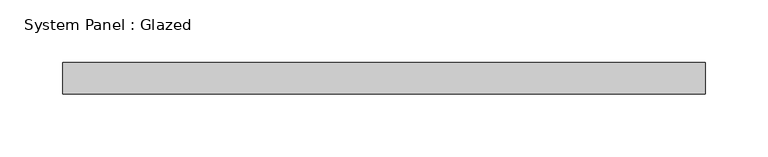
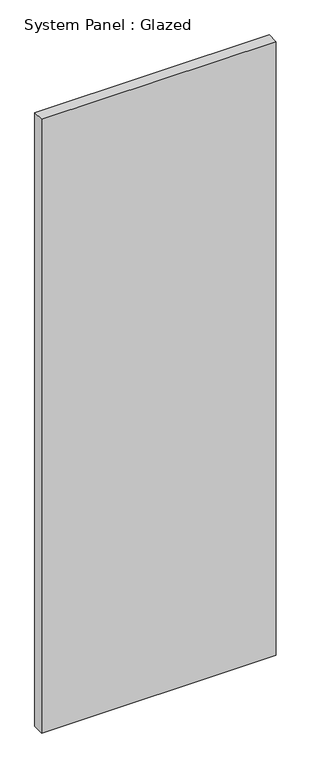
"""IFC4 building model written with IfcOpenShell, lengths in millimetres: plate geometry, System Panel : Glazed."""

from ifc_helpers import new_model, si_unit, origin, origin_with_axes, place, context, project, spatial, polyline, outline, extrude, source, transform, mapped, element, save


def system_panel_glazed_57bc90b1(model_context):
    return source(origin(), model_context, "Body", "SweptSolid", [
        extrude(outline(polyline([(257.175, 19.05), (-257.175, 19.05), (-257.175, 44.45), (257.175, 44.45), (257.175, 19.05)])), origin_with_axes(), (0.0, 0.0, 1.0), 1422.4),
    ])


if __name__ == "__main__":
    model = new_model("IFC4")
    model_context = context("Model", 3, world=origin())
    ifc_project = project(units=[si_unit("LENGTHUNIT", "METRE", prefix="MILLI")], contexts=[model_context])
    site = spatial("IfcSite", under=ifc_project)
    building = spatial("IfcBuilding", under=site)
    placement = place(None, origin())
    system_panel_glazed_shape = system_panel_glazed_57bc90b1(model_context)
    element("IfcPlate", 1, ObjectType="System Panel : Glazed", at=placement, inside=building, context=model_context, shape_type="MappedRepresentation", body=[
        mapped(system_panel_glazed_shape, transform((0.0, 0.0, 0.0), x_axis=(1.0, 0.0, 0.0), y_axis=(0.0, 1.0, 0.0), z_axis=(0.0, 0.0, 1.0))),
    ])
    save(model, "model.ifc")

# Revit data of these elements
# Type "System Panel : Glazed"
#   Construction Type Id = "GSP4R"
#   Analytic Construction = "1/8 in Pilkington single glazing"
#   Visual Light Transmittance = 0.9
#   Solar Heat Gain Coefficient = 0.86
#   Heat Transfer Coefficient (U) = 1.18115 BTU/(h·ft²·°F)
#   Define Thermal Properties by = 1
# Element 1 (IfcPlate, "System Panel : Glazed")
#   Materials on its faces: "Glass"
# Materials
#   "Glass": class "Glass", colour RGB 0 128 192, transparency 0.75, Description = "Soda Lime Glass", Cost = 0
